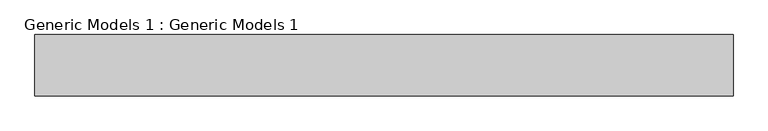
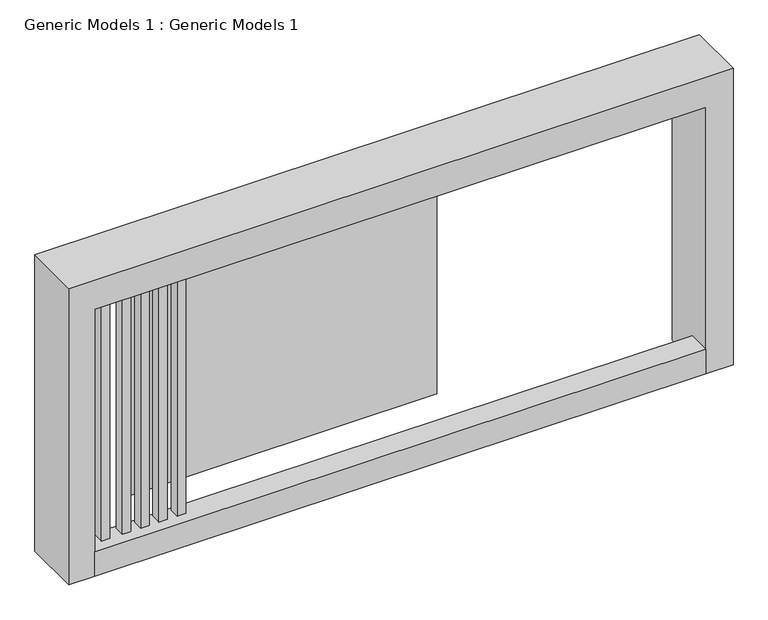
"""IFC4 building model written with IfcOpenShell, lengths in millimetres: proxy geometry, Generic Models 1 : Generic Models 1."""

from ifc_helpers import new_model, si_unit, frame, origin, place, context, project, spatial, polyline, outline, extrude, source, transform, mapped, element, save


def generic_models_1_generic_models_1_fa73b27a(model_context):
    return source(origin(), model_context, "Body", "SweptSolid", [
        extrude(outline(polyline([(-8657.4981007, 4426.1801686), (-11724.5481007, 4426.1801686), (-11724.5481007, 4427.4700124), (-8657.4981007, 4427.4700124), (-8657.4981007, 4426.1801686)])), frame((0.0, 0.0, -355.6), z_axis=(0.0, 0.0, 1.0), x_axis=(1.0, 0.0, 0.0)), (0.0, 0.0, 1.0), 2476.8472339),
        extrude(outline(polyline([(-11452.1827487, 3960.9431017), (-11452.1827487, 4062.5431017), (-11368.9481007, 4062.5431017), (-11368.9481007, 3960.9431017), (-11452.1827487, 3960.9431017)])), frame((0.0, 0.0, -355.6), z_axis=(0.0, 0.0, 1.0), x_axis=(1.0, 0.0, 0.0)), (0.0, 0.0, 1.0), 2489.2),
        extrude(outline(polyline([(-11629.9827487, 3960.9431017), (-11629.9827487, 4062.5431017), (-11546.7481007, 4062.5431017), (-11546.7481007, 3960.9431017), (-11629.9827487, 3960.9431017)])), frame((0.0, 0.0, -355.6), z_axis=(0.0, 0.0, 1.0), x_axis=(1.0, 0.0, 0.0)), (0.0, 0.0, 1.0), 2489.2),
        extrude(outline(polyline([(-11807.7827487, 3960.9431017), (-11807.7827487, 4062.5431017), (-11724.5481007, 4062.5431017), (-11724.5481007, 3960.9431017), (-11807.7827487, 3960.9431017)])), frame((0.0, 0.0, -355.6), z_axis=(0.0, 0.0, 1.0), x_axis=(1.0, 0.0, 0.0)), (0.0, 0.0, 1.0), 2489.2),
        extrude(outline(polyline([(-11985.5827487, 3960.9431017), (-11985.5827487, 4062.5431017), (-11902.3481007, 4062.5431017), (-11902.3481007, 3960.9431017), (-11985.5827487, 3960.9431017)])), frame((0.0, 0.0, -355.6), z_axis=(0.0, 0.0, 1.0), x_axis=(1.0, 0.0, 0.0)), (0.0, 0.0, 1.0), 2489.2),
        extrude(outline(polyline([(-12188.7827487, 3960.9431017), (-12188.7827487, 4062.5431017), (-12105.5481007, 4062.5431017), (-12105.5481007, 3960.9431017), (-12188.7827487, 3960.9431017)])), frame((0.0, 0.0, -355.6), z_axis=(0.0, 0.0, 1.0), x_axis=(1.0, 0.0, 0.0)), (0.0, 0.0, 1.0), 2489.2),
        extrude(outline(polyline([(-6368.7338554, 4090.3849429), (-6368.7338554, 3858.0110682), (-12312.3338554, 3858.0110682), (-12312.3338554, 4090.3849429), (-6368.7338554, 4090.3849429)])), frame((0.0, 0.0, -609.6), z_axis=(0.0, 0.0, 1.0), x_axis=(1.0, 0.0, 0.0)), (0.0, 0.0, 1.0), 254.0),
        extrude(outline(polyline([(2133.6, -6368.7338554), (-609.6, -6368.7338554), (-609.6, -6104.7981007), (2438.4, -6104.7981007), (2438.4, -12566.3338554), (-609.6, -12566.3338554), (-609.6, -12312.3338554), (2133.6, -12312.3338554), (2133.6, -6368.7338554)])), frame((0.0, 3858.0110682, 0.0), z_axis=(0.0, 1.0, 0.0), x_axis=(0.0, 0.0, 1.0)), (0.0, 0.0, 1.0), 569.4589441),
    ])


if __name__ == "__main__":
    model = new_model("IFC4")
    model_context = context("Model", 3, world=origin())
    ifc_project = project(units=[si_unit("LENGTHUNIT", "METRE", prefix="MILLI")], contexts=[model_context])
    site = spatial("IfcSite", under=ifc_project)
    building = spatial("IfcBuilding", under=site)
    placement = place(None, origin())
    generic_models_1_generic_models_1_shape = generic_models_1_generic_models_1_fa73b27a(model_context)
    element("IfcBuildingElementProxy", 1, Name="Generic Models 1 : Generic Models 1", ObjectType="Generic Models 1 : Generic Models 1", at=placement, inside=building, context=model_context, shape_type="MappedRepresentation", body=[
        mapped(generic_models_1_generic_models_1_shape, transform((0.0, 0.0, 0.0), x_axis=(1.0, 0.0, 0.0), y_axis=(0.0, 1.0, 0.0), z_axis=(0.0, 0.0, 1.0))),
    ])
    save(model, "model.ifc")
